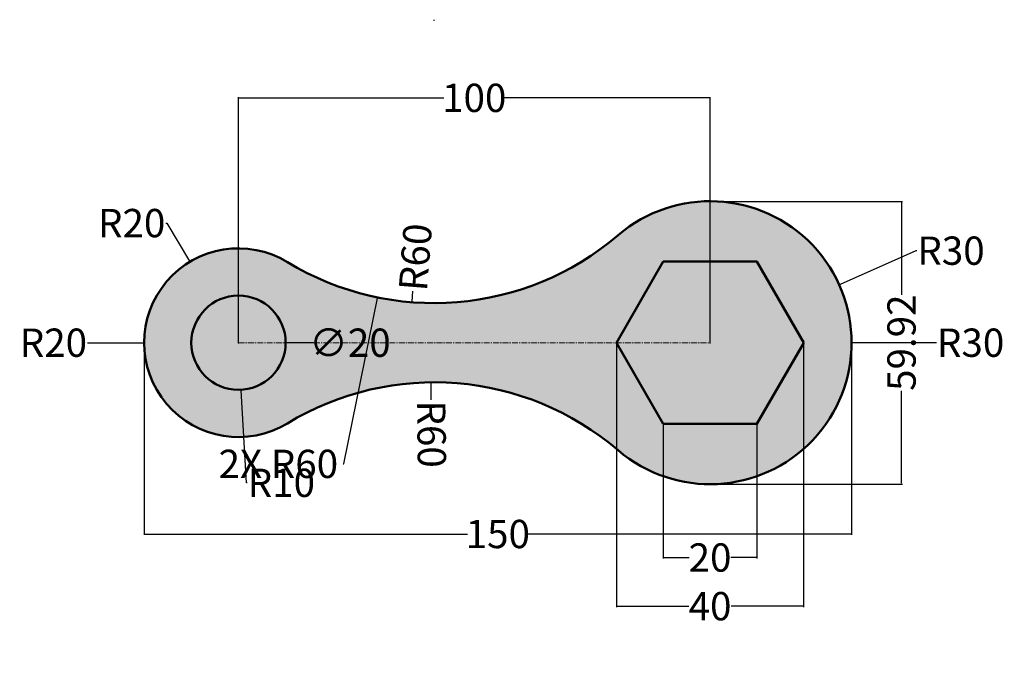
# Model space of a CAD drawing. Units: millimetres. Extents: x -9 to 200, y -5 to 132.
import ezdxf

# ---------------------------------------------------------------- set-up
doc = ezdxf.new("R2010")
doc.units = ezdxf.units.MM
doc.header["$MEASUREMENT"] = 0
doc.linetypes.add('CENTER', pattern=[2, 1.25, -0.25, 0.25, -0.25])
for name, color, linetype, lineweight in [('M-CNTR', 4, 'CENTER', 18), ('M-DIMS', 2, 'Continuous', 25), ('M-HATC', 252, 'Continuous', 18), ('M-OUTL', 7, 'Continuous', 50)]:
    doc.layers.add(name, color=color, linetype=linetype, lineweight=lineweight)
doc.styles.get("Standard").update_dxf_attribs({"font": 'arial.ttf'})
doc.dimstyles.get("Standard").update_dxf_attribs({"dimtxt": 6, "dimasz": 0.18, "dimexe": 0.18, "dimexo": 0.0625, "dimgap": 0.09, "dimtad": 0, "dimtoh": 1, "dimdec": 0, "dimzin": 0, "dimdsep": 46, "dimtxsty": 'Standard', "dimcen": 0.09, "dimadec": 0, "dimazin": 0, "dimtfac": 1, "dimtdec": 0, "dimtofl": 0, "dimtmove": 0, "dimatfit": 3, "dimfxl": 1, "dimtolj": 1, "dimtzin": 0, "dimarcsym": 0})

# ---------------------------------------------------------------- blocks, each defined once
blk = doc.blocks.new('*D1')
at = {"layer": 'Defpoints', "color": 0, "transparency": 16777216}
for p in [(137.48, 115.48), (37.48, 63.57), (137.48, 63.57)]:
    blk.add_point(p, dxfattribs=at)
at = {"layer": 'M-DIMS', "color": 0, "lineweight": -2, "transparency": 16777216}
for p, q in [((37.48, 63.63), (37.48, 115.66)), ((37.66, 115.48), (81.06, 115.48)), ((137.3, 115.48), (93.91, 115.48)), ((137.48, 63.63), (137.48, 115.66))]:
    blk.add_line(p, q, dxfattribs=at)
at = {"layer": 'M-DIMS', "color": 0, "transparency": 16777216}
for points in [[(37.66, 115.51), (37.66, 115.45), (37.48, 115.48)], [(137.3, 115.51), (137.3, 115.45), (137.48, 115.48)]]:
    blk.add_solid(points, dxfattribs=at)
at = {"layer": 'M-DIMS', "color": 0, "transparency": 16777216, "insert": (87.48, 115.48), "char_height": 6, "attachment_point": 5}
blk.add_mtext('\\A1;100', dxfattribs=at)
blk = doc.blocks.new('*D2')
at = {"layer": 'Defpoints', "color": 0, "transparency": 16777216}
for p in [(164.87, 75.81), (137.48, 63.57)]:
    blk.add_point(p, dxfattribs=at)
at = {"layer": 'M-DIMS', "color": 0, "lineweight": -2, "transparency": 16777216}
for p, q in [((181.14, 83.08), (165.04, 75.88)), ((181.32, 83.08), (181.14, 83.08)), ((137.39, 63.57), (137.57, 63.57)), ((137.48, 63.48), (137.48, 63.66))]:
    blk.add_line(p, q, dxfattribs=at)
at = {"layer": 'M-DIMS', "color": 0, "transparency": 16777216}
blk.add_solid([(165.03, 75.91), (165.05, 75.85), (164.87, 75.81)], dxfattribs=at)
at = {"layer": 'M-DIMS', "color": 0, "transparency": 16777216, "insert": (188.57, 83.08), "char_height": 6, "attachment_point": 5}
blk.add_mtext('\\A1;R30', dxfattribs=at)
blk = doc.blocks.new('*D3')
at = {"layer": 'Defpoints', "color": 0, "transparency": 16777216}
for p in [(78.98, 131.96), (74.24, 72.15)]:
    blk.add_point(p, dxfattribs=at)
at = {"layer": 'M-DIMS', "color": 0, "lineweight": -2, "transparency": 16777216}
blk.add_line((74.42, 74.48), (74.25, 72.33), dxfattribs=at)
at = {"layer": 'M-DIMS', "color": 0, "transparency": 16777216}
blk.add_solid([(74.22, 72.33), (74.28, 72.33), (74.24, 72.15)], dxfattribs=at)
at = {"layer": 'M-DIMS', "color": 0, "transparency": 16777216, "insert": (75, 81.7), "char_height": 6, "attachment_point": 5, "rotation": 85.4629}
blk.add_mtext('\\A1;R60', dxfattribs=at)
blk = doc.blocks.new('*D4')
at = {"layer": 'Defpoints', "color": 0, "transparency": 16777216}
for p in [(78.32, 55.17), (78.98, -4.83)]:
    blk.add_point(p, dxfattribs=at)
at = {"layer": 'M-DIMS', "color": 0, "lineweight": -2, "transparency": 16777216}
blk.add_line((78.36, 51.44), (78.32, 54.99), dxfattribs=at)
at = {"layer": 'M-DIMS', "color": 0, "transparency": 16777216}
blk.add_solid([(78.35, 54.99), (78.29, 54.99), (78.32, 55.17)], dxfattribs=at)
at = {"layer": 'M-DIMS', "color": 0, "transparency": 16777216, "insert": (78.44, 44.19), "char_height": 6, "attachment_point": 5, "rotation": 270.6334}
blk.add_mtext('\\A1;R60', dxfattribs=at)
blk = doc.blocks.new('*D5')
at = {"layer": 'Defpoints', "color": 0, "transparency": 16777216}
for p in [(27.2, 80.72), (37.48, 63.57)]:
    blk.add_point(p, dxfattribs=at)
at = {"layer": 'M-DIMS', "color": 0, "lineweight": -2, "transparency": 16777216}
for p, q in [((22.09, 88.93), (22.27, 88.93)), ((22.27, 88.93), (27.1, 80.87)), ((37.39, 63.57), (37.57, 63.57)), ((37.48, 63.48), (37.48, 63.66))]:
    blk.add_line(p, q, dxfattribs=at)
at = {"layer": 'M-DIMS', "color": 0, "transparency": 16777216}
blk.add_solid([(27.13, 80.89), (27.08, 80.86), (27.2, 80.72)], dxfattribs=at)
at = {"layer": 'M-DIMS', "color": 0, "transparency": 16777216, "insert": (14.84, 88.93), "char_height": 6, "attachment_point": 5}
blk.add_mtext('\\A1;R20', dxfattribs=at)
blk = doc.blocks.new('*D6')
at = {"layer": 'Defpoints', "color": 0, "transparency": 16777216}
for p in [(37.48, 63.57), (38.05, 53.58)]:
    blk.add_point(p, dxfattribs=at)
at = {"layer": 'M-DIMS', "color": 0, "lineweight": -2, "transparency": 16777216}
for p, q in [((37.39, 63.57), (37.57, 63.57)), ((37.48, 63.48), (37.48, 63.66)), ((39.16, 33.86), (38.06, 53.4)), ((39.34, 33.86), (39.16, 33.86))]:
    blk.add_line(p, q, dxfattribs=at)
at = {"layer": 'M-DIMS', "color": 0, "transparency": 16777216}
blk.add_solid([(38.09, 53.4), (38.03, 53.4), (38.05, 53.58)], dxfattribs=at)
at = {"layer": 'M-DIMS', "color": 0, "transparency": 16777216, "insert": (46.58, 33.86), "char_height": 6, "attachment_point": 5}
blk.add_mtext('\\A1;R10', dxfattribs=at)
blk = doc.blocks.new('*D7')
at = {"layer": 'Defpoints', "color": 0, "transparency": 16777216}
for p in [(117.64, 63.57), (157.33, 63.57), (157.33, 7.71)]:
    blk.add_point(p, dxfattribs=at)
at = {"layer": 'M-DIMS', "color": 0, "lineweight": -2, "transparency": 16777216}
for p, q in [((117.64, 63.5), (117.64, 7.53)), ((157.33, 63.5), (157.33, 7.53)), ((117.82, 7.71), (132.99, 7.71)), ((157.15, 7.71), (141.98, 7.71))]:
    blk.add_line(p, q, dxfattribs=at)
at = {"layer": 'M-DIMS', "color": 0, "transparency": 16777216}
for points in [[(117.82, 7.74), (117.82, 7.68), (117.64, 7.71)], [(157.15, 7.74), (157.15, 7.68), (157.33, 7.71)]]:
    blk.add_solid(points, dxfattribs=at)
at = {"layer": 'M-DIMS', "color": 0, "transparency": 16777216, "insert": (137.48, 7.71), "char_height": 6, "attachment_point": 5}
blk.add_mtext('\\A1;40', dxfattribs=at)
blk = doc.blocks.new('*D8')
at = {"layer": 'Defpoints', "color": 0, "transparency": 16777216}
for p in [(127.56, 46.38), (147.41, 46.38), (147.41, 18.03)]:
    blk.add_point(p, dxfattribs=at)
at = {"layer": 'M-DIMS', "color": 0, "lineweight": -2, "transparency": 16777216}
for p, q in [((127.56, 46.32), (127.56, 17.85)), ((147.41, 46.32), (147.41, 17.85)), ((127.74, 18.03), (133.06, 18.03)), ((147.23, 18.03), (141.91, 18.03))]:
    blk.add_line(p, q, dxfattribs=at)
at = {"layer": 'M-DIMS', "color": 0, "transparency": 16777216}
for points in [[(127.74, 18.06), (127.74, 18), (127.56, 18.03)], [(147.23, 18.06), (147.23, 18), (147.41, 18.03)]]:
    blk.add_solid(points, dxfattribs=at)
at = {"layer": 'M-DIMS', "color": 0, "transparency": 16777216, "insert": (137.48, 18.03), "char_height": 6, "attachment_point": 5}
blk.add_mtext('\\A1;20', dxfattribs=at)
blk = doc.blocks.new('*D9')
at = {"layer": 'Defpoints', "color": 0, "transparency": 16777216}
for p in [(17.48, 63.57), (167.48, 63.57), (167.48, 23.01)]:
    blk.add_point(p, dxfattribs=at)
at = {"layer": 'M-DIMS', "color": 0, "lineweight": -2, "transparency": 16777216}
for p, q in [((17.48, 63.5), (17.48, 22.83)), ((167.48, 63.5), (167.48, 22.83)), ((17.66, 23.01), (86.06, 23.01)), ((167.3, 23.01), (98.91, 23.01))]:
    blk.add_line(p, q, dxfattribs=at)
at = {"layer": 'M-DIMS', "color": 0, "transparency": 16777216}
for points in [[(17.66, 23.04), (17.66, 22.98), (17.48, 23.01)], [(167.3, 23.04), (167.3, 22.98), (167.48, 23.01)]]:
    blk.add_solid(points, dxfattribs=at)
at = {"layer": 'M-DIMS', "color": 0, "transparency": 16777216, "insert": (92.48, 23.01), "char_height": 6, "attachment_point": 5}
blk.add_mtext('\\A1;150', dxfattribs=at)
blk = doc.blocks.new('*D10')
at = {"layer": 'Defpoints', "color": 0, "transparency": 16777216}
for p in [(139.04, 93.53), (178.08, 93.53), (139.04, 33.61)]:
    blk.add_point(p, dxfattribs=at)
at = {"layer": 'M-DIMS', "color": 0, "lineweight": -2, "transparency": 16777216}
for p, q in [((139.1, 93.53), (178.26, 93.53)), ((178.08, 93.35), (178.08, 73.75)), ((178.08, 33.79), (178.08, 53.38)), ((139.1, 33.61), (178.26, 33.61))]:
    blk.add_line(p, q, dxfattribs=at)
at = {"layer": 'M-DIMS', "color": 0, "transparency": 16777216}
for points in [[(178.05, 93.35), (178.11, 93.35), (178.08, 93.53)], [(178.05, 33.79), (178.11, 33.79), (178.08, 33.61)]]:
    blk.add_solid(points, dxfattribs=at)
at = {"layer": 'M-DIMS', "color": 0, "transparency": 16777216, "insert": (178.08, 63.57), "char_height": 6, "attachment_point": 5, "rotation": 90}
blk.add_mtext('\\A1;59.92', dxfattribs=at)
blk = doc.blocks.new('*D11')
at = {"layer": 'Defpoints', "color": 0, "transparency": 16777216}
for p in [(17.48, 63.57), (37.48, 63.57)]:
    blk.add_point(p, dxfattribs=at)
at = {"layer": 'M-DIMS', "color": 0, "lineweight": -2, "transparency": 16777216}
for p, q in [((5.48, 63.57), (17.3, 63.57)), ((37.39, 63.57), (37.57, 63.57)), ((37.48, 63.48), (37.48, 63.66))]:
    blk.add_line(p, q, dxfattribs=at)
at = {"layer": 'M-DIMS', "color": 0, "transparency": 16777216}
blk.add_solid([(17.3, 63.6), (17.3, 63.54), (17.48, 63.57)], dxfattribs=at)
at = {"layer": 'M-DIMS', "color": 0, "transparency": 16777216, "insert": (-1.76, 63.57), "char_height": 6, "attachment_point": 5}
blk.add_mtext('\\A1;R20', dxfattribs=at)
blk = doc.blocks.new('*D12')
at = {"layer": 'Defpoints', "color": 0, "transparency": 16777216}
for p in [(137.48, 63.57), (167.48, 63.57)]:
    blk.add_point(p, dxfattribs=at)
at = {"layer": 'M-DIMS', "color": 0, "lineweight": -2, "transparency": 16777216}
for p, q in [((137.39, 63.57), (137.57, 63.57)), ((137.48, 63.48), (137.48, 63.66)), ((185.48, 63.57), (167.66, 63.57))]:
    blk.add_line(p, q, dxfattribs=at)
at = {"layer": 'M-DIMS', "color": 0, "transparency": 16777216}
blk.add_solid([(167.66, 63.6), (167.66, 63.54), (167.48, 63.57)], dxfattribs=at)
at = {"layer": 'M-DIMS', "color": 0, "transparency": 16777216, "insert": (192.73, 63.57), "char_height": 6, "attachment_point": 5}
blk.add_mtext('\\A1;R30', dxfattribs=at)
blk = doc.blocks.new('*D13')
at = {"layer": 'Defpoints', "color": 0, "transparency": 16777216}
for p in [(27.48, 63.57), (47.48, 63.57)]:
    blk.add_point(p, dxfattribs=at)
at = {"layer": 'M-DIMS', "color": 0, "lineweight": -2, "transparency": 16777216}
for p, q in [((37.39, 63.57), (37.57, 63.57)), ((37.48, 63.48), (37.48, 63.66)), ((53.48, 63.57), (47.66, 63.57))]:
    blk.add_line(p, q, dxfattribs=at)
at = {"layer": 'M-DIMS', "color": 0, "transparency": 16777216}
blk.add_solid([(47.66, 63.6), (47.66, 63.54), (47.48, 63.57)], dxfattribs=at)
at = {"layer": 'M-DIMS', "color": 0, "transparency": 16777216, "insert": (61.13, 63.57), "char_height": 6, "attachment_point": 5}
blk.add_mtext('\\A1;∅20', dxfattribs=at)
blk = doc.blocks.new('*D14')
at = {"layer": 'Defpoints', "color": 0, "transparency": 16777216}
for p in [(78.98, 131.96), (67.03, 73.16)]:
    blk.add_point(p, dxfattribs=at)
at = {"layer": 'M-DIMS', "color": 0, "lineweight": -2, "transparency": 16777216}
for p, q in [((78.89, 131.96), (79.07, 131.96)), ((78.98, 131.87), (78.98, 132.05)), ((59.86, 37.88), (67, 72.99)), ((59.68, 37.88), (59.86, 37.88))]:
    blk.add_line(p, q, dxfattribs=at)
at = {"layer": 'M-DIMS', "color": 0, "transparency": 16777216}
blk.add_solid([(66.97, 72.99), (67.03, 72.98), (67.03, 73.16)], dxfattribs=at)
at = {"layer": 'M-DIMS', "color": 0, "transparency": 16777216, "insert": (45.94, 37.88), "char_height": 6, "attachment_point": 5}
blk.add_mtext('\\A1;2X R60', dxfattribs=at)

msp = doc.modelspace()

# ---------------------------------------------------------------- hatches: boundary and pattern name
at = {"layer": 'M-HATC'}
h = msp.add_hatch(color=256, dxfattribs=at)
h.set_gradient(color1=(255, 0, 255), color2=(248, 153, 30))
h.paths.add_polyline_path([(47.86, 46.468, -0.3239072), (117.985, 40.768, 2.1712406), (117.985, 86.364, -0.3239072), (47.86, 80.665, 1.7764696)])
h.paths.add_polyline_path([(47.485, 63.566), (117.639, 63.566), (127.562, 80.753), (147.408, 80.753), (157.331, 63.566), (147.408, 46.379), (127.562, 46.379), (117.639, 63.566), (47.485, 63.566, -1), (27.485, 63.566, -1)], flags=16)
h = msp.add_hatch(color=256, dxfattribs=at)
h.set_gradient(color1=(0, 255, 0), color2=(255, 255, 0), name='CYLINDER')
h.paths.add_polyline_path([(27.485, 63.566, 1), (47.485, 63.566, 1)])
h.paths.add_polyline_path([(127.562, 80.753), (117.639, 63.566), (127.562, 46.379), (147.408, 46.379), (157.331, 63.566), (147.408, 80.753)])

# ---------------------------------------------------------------- linework, layer by layer
at = {"layer": 'M-CNTR'}
msp.add_line((37.485, 63.566), (137.485, 63.566), dxfattribs=at)
at = {"layer": 'M-OUTL'}
msp.add_lwpolyline([(47.86, 80.665, 0.3239072), (117.985, 86.364, -2.1712406), (117.985, 40.768, 0.3239072), (47.86, 46.468, -1.7764696)], format="xyb", close=True, dxfattribs=at)
msp.add_lwpolyline([(157.331, 63.566), (147.408, 80.753), (127.562, 80.753), (117.639, 63.566), (127.562, 46.379), (147.408, 46.379)], close=True, dxfattribs=at)
msp.add_circle((37.485, 63.566), 10, dxfattribs=at)

# ---------------------------------------------------------------- dimensions: what is measured, and where the dimension line sits
at = {"layer": 'M-DIMS'}
dim = msp.add_radius_dim(center=(78.985, 131.96), mpoint=(67.033, 73.163), text='2X <>', dimstyle='Standard', override={"dimdec": 0, "dimlfac": 1, "dimrnd": 0, "dimzin": 0, "dimdsep": 46, "dimlunit": 2}, dxfattribs=at)
dim.commit()
dim.dimension.update_dxf_attribs({"geometry": '*D14', "text_midpoint": (45.936, 37.884), "dimtype": 164})
for center, mpoint, override, picture, middle in [((78.985, 131.96), (74.239, 72.148), {"dimclrd": 0, "dimclre": 0, "dimclrt": 0}, '*D3', (74.997, 81.702)), ((37.485, 63.566), (27.196, 80.717), {"dimclrd": 0, "dimclre": 0, "dimclrt": 0}, '*D5', (14.841, 88.929)), ((137.485, 63.566), (164.874, 75.808), {"dimclrd": 0, "dimclre": 0, "dimclrt": 0}, '*D2', (188.57, 83.079)), ((37.485, 63.566), (17.485, 63.566), {"dimdec": 0, "dimlfac": 1, "dimrnd": 0, "dimzin": 0, "dimdsep": 46, "dimlunit": 2}, '*D11', (5.485, 63.566)), ((137.485, 63.566), (167.485, 63.566), {"dimdec": 0, "dimlfac": 1, "dimrnd": 0, "dimzin": 0, "dimdsep": 46, "dimlunit": 2}, '*D12', (185.485, 63.566)), ((37.485, 63.566), (38.046, 53.582), {"dimclrd": 0, "dimclre": 0, "dimclrt": 0}, '*D6', (46.584, 33.865)), ((78.985, -4.828), (78.322, 55.168), {"dimclrd": 0, "dimclre": 0, "dimclrt": 0}, '*D4', (78.443, 44.189))]:
    dim = msp.add_radius_dim(center=center, mpoint=mpoint, dimstyle='Standard', override=override, dxfattribs=at)
    dim.commit()
    dim.dimension.update_dxf_attribs({"geometry": picture, "text_midpoint": middle, "dimtype": 164})
for base, p1, p2, override, picture, middle in [((137.485, 115.479), (37.485, 63.566), (137.485, 63.566), {"dimclrd": 0, "dimclre": 0, "dimclrt": 0}, '*D1', (87.485, 115.479)), ((167.485, 23.007), (17.485, 63.566), (167.485, 63.566), {"dimdec": 0, "dimlfac": 1, "dimrnd": 0, "dimzin": 0, "dimdsep": 46, "dimlunit": 2}, '*D9', (92.485, 23.007)), ((157.331, 7.709), (117.639, 63.566), (157.331, 63.566), {"dimclrd": 0, "dimclre": 0, "dimclrt": 0}, '*D7', (137.485, 7.709)), ((147.408, 18.034), (127.562, 46.379), (147.408, 46.379), {"dimclrd": 0, "dimclre": 0, "dimclrt": 0}, '*D8', (137.485, 18.034))]:
    dim = msp.add_linear_dim(base=base, p1=p1, p2=p2, dimstyle='Standard', override=override, dxfattribs=at)
    dim.commit()
    dim.dimension.update_dxf_attribs({"geometry": picture, "text_midpoint": middle})
dim = msp.add_linear_dim(base=(178.085, 93.526), p1=(139.04, 33.607), p2=(139.04, 93.526), angle=90, dimstyle='Standard', override={"dimdec": 2, "dimlfac": 1, "dimrnd": 0, "dimzin": 0, "dimdsep": 46, "dimlunit": 2}, dxfattribs=at)
dim.commit()
dim.dimension.update_dxf_attribs({"geometry": '*D10', "text_midpoint": (178.085, 63.566)})
dim = msp.add_diameter_dim_2p(p1=(27.485, 63.566), p2=(47.485, 63.566), dimstyle='Standard', override={"dimdec": 0, "dimlfac": 1, "dimrnd": 0, "dimzin": 0, "dimdsep": 46, "dimlunit": 2}, dxfattribs=at)
dim.commit()
dim.dimension.update_dxf_attribs({"geometry": '*D13', "text_midpoint": (53.485, 63.566), "dimtype": 163})

doc.saveas('drawing.dxf')
